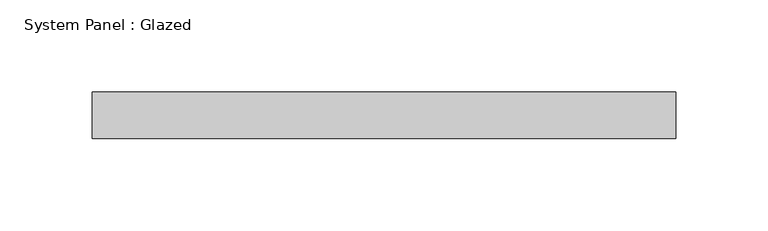
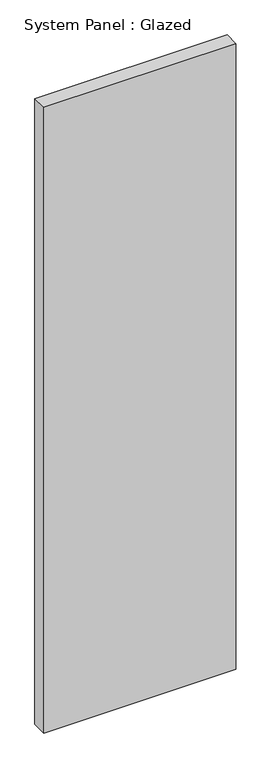
"""IFC4 building model written with IfcOpenShell, lengths in millimetres: plate geometry, System Panel : Glazed."""

from ifc_helpers import new_model, si_unit, origin, origin_with_axes, place, context, project, spatial, polyline, outline, extrude, source, transform, mapped, element, save


def system_panel_glazed_e0d10779(model_context):
    return source(origin(), model_context, "Body", "SweptSolid", [
        extrude(outline(polyline([(158.5603194, 19.05), (-158.5603194, 19.05), (-158.5603194, 44.45), (158.5603194, 44.45), (158.5603194, 19.05)])), origin_with_axes(), (0.0, 0.0, 1.0), 1092.2),
    ])


if __name__ == "__main__":
    model = new_model("IFC4")
    model_context = context("Model", 3, world=origin())
    ifc_project = project(units=[si_unit("LENGTHUNIT", "METRE", prefix="MILLI")], contexts=[model_context])
    site = spatial("IfcSite", under=ifc_project)
    building = spatial("IfcBuilding", under=site)
    placement = place(None, origin())
    system_panel_glazed_shape = system_panel_glazed_e0d10779(model_context)
    element("IfcPlate", 1, ObjectType="System Panel : Glazed", at=placement, inside=building, context=model_context, shape_type="MappedRepresentation", body=[
        mapped(system_panel_glazed_shape, transform((0.0, 0.0, 0.0), x_axis=(1.0, 0.0, 0.0), y_axis=(0.0, 1.0, 0.0), z_axis=(0.0, 0.0, 1.0))),
    ])
    save(model, "model.ifc")

# Revit data of these elements
# Type "System Panel : Glazed"
#   Construction Type Id = "GSP4R"
#   Analytic Construction = "1/8 in Pilkington single glazing"
#   Visual Light Transmittance = 0.9
#   Solar Heat Gain Coefficient = 0.86
#   Heat Transfer Coefficient (U) = 1.18115 BTU/(h·ft²·°F)
# Element 1 (IfcPlate, "System Panel : Glazed")
#   Materials on its faces: "Glass"
# Materials
#   "Glass": class "Glass", colour RGB 0 128 192, transparency 0.75, Description = "Soda Lime Glass", Cost = 0
